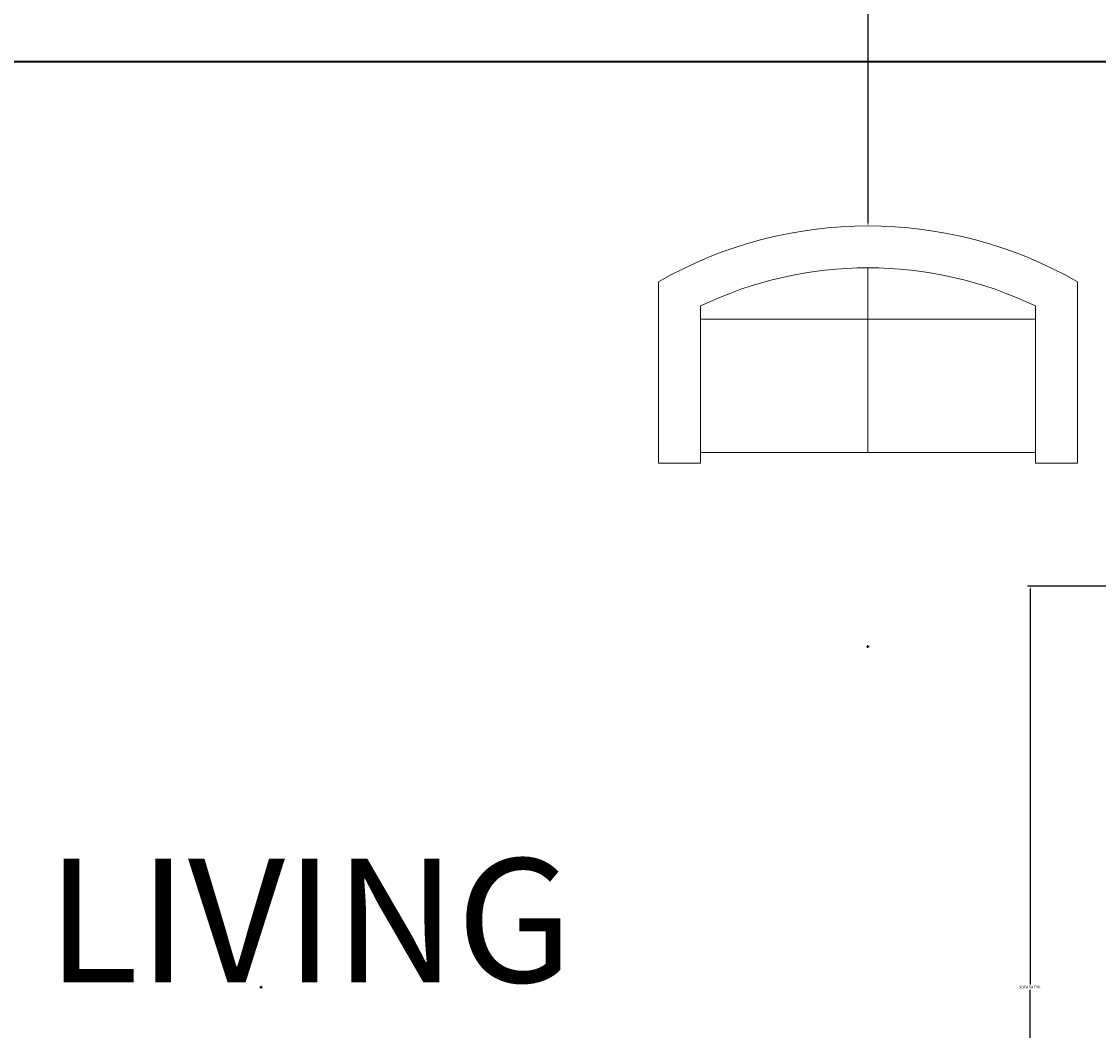
# Model space of a CAD drawing. Units: feet. Extents: x 1654 to 2985, y 1348 to 2230.
# Tile 36 of 53: x 2100 to 2173, y 1821 to 1889. Entities that reach past the tile are written whole.
import ezdxf

# ---------------------------------------------------------------- set-up
doc = ezdxf.new("R2010")
doc.units = ezdxf.units.FT
for name, color, linetype, lineweight in [('A-ANNO-DIMS', 2, 'Continuous', 18), ('A-AREA-IDEN', 7, 'Continuous', 18), ('A-FURN', 8, 'Continuous', 13), ('A-WALL', 7, 'Continuous', 35)]:
    doc.layers.add(name, color=color, linetype=linetype, lineweight=lineweight)
doc.styles.get("Standard").update_dxf_attribs({"font": 'arial.ttf'})
doc.dimstyles.get("Standard").update_dxf_attribs({"dimtxt": 0.18, "dimasz": 0.18, "dimexe": 0.18, "dimexo": 0.0625, "dimgap": 0.09, "dimtad": 0, "dimtih": 1, "dimtoh": 1, "dimdec": 4, "dimzin": 0, "dimdsep": 46, "dimtxsty": 'Standard', "dimcen": 0.09, "dimadec": 0, "dimazin": 0, "dimtfac": 1, "dimtdec": 4, "dimtofl": 0, "dimtmove": 0, "dimatfit": 3, "dimfxl": 1, "dimtolj": 1, "dimtzin": 0, "dimarcsym": 0})

# ---------------------------------------------------------------- blocks, each defined once
blk = doc.blocks.new('Sofa - Roundback Loveseat 5 ft.')
for p, q in [((0, -32.44198), (0, -5.99998)), ((-24, -33.99998), (-24, -11.46958)), ((24.00004, -33.99998), (24.00004, -11.46958)), ((-23.9998, -13.38178), (23.99986, -13.38178)), ((-24, -32.44198), (24.00004, -32.44198))]:
    blk.add_line(p, q)
for points in [[(-24, -33.99998), (-30, -33.99998), (-30, -7.99998)], [(30.00004, -7.99998), (30.00004, -33.99998), (24.00004, -33.99998)]]:
    blk.add_lwpolyline(points)
for centre, radius, start, end in [((0, -60.24998), 60.24998, 60.13715, 119.8628), ((0, -61.38438), 55.38444, 64.32083, 115.6792)]:
    blk.add_arc(centre, radius, start, end)
blk = doc.blocks.new('*D38')
at = {"layer": 'A-ANNO-DIMS', "color": 0, "lineweight": -2, "transparency": 16777216}
for p, q in [((2176.839, 1850.733), (2168.575, 1850.733)), ((2168.755, 1850.553), (2168.755, 1823.764)), ((2168.755, 1796.609), (2168.755, 1823.398)), ((2176.839, 1796.429), (2168.575, 1796.429))]:
    blk.add_line(p, q, dxfattribs=at)
at = {"layer": 'A-ANNO-DIMS', "color": 0, "transparency": 16777216}
for points in [[(2168.725, 1850.553), (2168.785, 1850.553), (2168.755, 1850.733)], [(2168.725, 1796.609), (2168.785, 1796.609), (2168.755, 1796.429)]]:
    blk.add_solid(points, dxfattribs=at)
at = {"layer": 'Defpoints', "color": 0, "transparency": 16777216}
for p in [(2176.901, 1850.733), (2168.755, 1796.429), (2176.901, 1796.429)]:
    blk.add_point(p, dxfattribs=at)
at = {"layer": 'A-ANNO-DIMS', "color": 0, "transparency": 16777216, "insert": (2168.755, 1823.581), "char_height": 0.18, "attachment_point": 5}
blk.add_mtext('\\A1;SOFA 54 TYP.', dxfattribs=at)
blk = doc.blocks.new('*D80')
at = {"layer": 'A-ANNO-DIMS', "color": 0, "lineweight": -2, "transparency": 16777216}
for p, q in [((2070.092, 2039.192), (2070.092, 1534.075)), ((2202.092, 2039.192), (2202.092, 1534.075)), ((2070.272, 1534.255), (2135.813, 1534.255)), ((2201.912, 1534.255), (2136.372, 1534.255))]:
    blk.add_line(p, q, dxfattribs=at)
at = {"layer": 'A-ANNO-DIMS', "color": 0, "transparency": 16777216}
for points in [[(2070.272, 1534.285), (2070.272, 1534.225), (2070.092, 1534.255)], [(2201.912, 1534.285), (2201.912, 1534.225), (2202.092, 1534.255)]]:
    blk.add_solid(points, dxfattribs=at)
at = {"layer": 'Defpoints', "color": 0, "transparency": 16777216}
for p in [(2070.092, 2039.255), (2202.092, 2039.255), (2202.092, 1534.255)]:
    blk.add_point(p, dxfattribs=at)
at = {"layer": 'A-ANNO-DIMS', "color": 0, "transparency": 16777216, "insert": (2136.092, 1534.255), "char_height": 0.18, "attachment_point": 5}
blk.add_mtext('\\A1;132', dxfattribs=at)
blk = doc.blocks.new('*D108')
at = {"layer": 'A-ANNO-DIMS', "color": 0, "lineweight": -2, "transparency": 16777216}
for p, q in [((2116.561, 1823.581), (2116.741, 1823.581)), ((2116.651, 1823.491), (2116.651, 1823.671)), ((2242.014, 1823.581), (2195.183, 1823.581))]:
    blk.add_line(p, q, dxfattribs=at)
at = {"layer": 'A-ANNO-DIMS', "color": 0, "transparency": 16777216}
blk.add_solid([(2195.183, 1823.611), (2195.183, 1823.551), (2195.003, 1823.581)], dxfattribs=at)
at = {"layer": 'Defpoints', "color": 0, "transparency": 16777216}
for p in [(2116.651, 1823.581), (2195.003, 1823.581)]:
    blk.add_point(p, dxfattribs=at)
at = {"layer": 'A-ANNO-DIMS', "color": 0, "transparency": 16777216, "insert": (2242.689, 1823.581), "char_height": 0.18, "attachment_point": 5}
blk.add_mtext('\\A1;2X R78.35', dxfattribs=at)
blk = doc.blocks.new('*D110')
at = {"layer": 'A-ANNO-DIMS', "color": 0, "lineweight": -2, "transparency": 16777216}
for p, q in [((2157.583, 1892.245), (2157.763, 1892.245)), ((2157.763, 1892.245), (2157.763, 1875.33)), ((2157.763, 1846.568), (2157.763, 1846.748)), ((2157.673, 1846.658), (2157.853, 1846.658))]:
    blk.add_line(p, q, dxfattribs=at)
at = {"layer": 'A-ANNO-DIMS', "color": 0, "transparency": 16777216}
blk.add_solid([(2157.793, 1875.33), (2157.733, 1875.33), (2157.763, 1875.15)], dxfattribs=at)
at = {"layer": 'Defpoints', "color": 0, "transparency": 16777216}
for p in [(2157.763, 1875.15), (2157.763, 1846.658)]:
    blk.add_point(p, dxfattribs=at)
at = {"layer": 'A-ANNO-DIMS', "color": 0, "transparency": 16777216, "insert": (2156.908, 1892.245), "char_height": 0.18, "attachment_point": 5}
blk.add_mtext('\\A1;2X R28.49', dxfattribs=at)

msp = doc.modelspace()

# ---------------------------------------------------------------- linework, layer by layer
at = {"layer": 'A-WALL'}
msp.add_line((2202.0924, 1886.2549), (2070.0924, 1886.2549), dxfattribs=at)

# ---------------------------------------------------------------- block references
at = {"layer": 'A-FURN', "xscale": 0.4728872769476647, "yscale": 0.4728872769476647, "zscale": 0.4728872769476647}
msp.add_blockref('Sofa - Roundback Loveseat 5 ft.', (2157.7631, 1875.1496), dxfattribs=at)

# ---------------------------------------------------------------- texts
at = {"layer": 'A-AREA-IDEN'}
msp.add_text('LIVING', height=8.38114, dxfattribs=at).set_placement((2102.1259, 1823.9066))

# ---------------------------------------------------------------- dimensions: what is measured, and where the dimension line sits
at = {"layer": 'A-ANNO-DIMS'}
dim = msp.add_linear_dim(base=(2202.0924, 1534.2549), p1=(2070.0924, 2039.2549), p2=(2202.0924, 2039.2549), dimstyle='Standard', override={"dimdec": 0, "dimlfac": 1, "dimrnd": 0, "dimzin": 0, "dimdsep": 46, "dimlunit": 2}, dxfattribs=at)
dim.commit()
dim.dimension.update_dxf_attribs({"geometry": '*D80', "text_midpoint": (2136.0924, 1534.2549)})
for center, mpoint, picture, middle in [((2157.7631, 1846.6582), (2157.763, 1875.1496), '*D110', (2156.908, 1892.2445)), ((2116.6507, 1823.581), (2195.0027, 1823.581), '*D108', (2242.0138, 1823.581))]:
    dim = msp.add_radius_dim(center=center, mpoint=mpoint, text='2X <>', dimstyle='Standard', override={"dimdec": 2, "dimlfac": 1, "dimrnd": 0, "dimzin": 0, "dimdsep": 46, "dimlunit": 2}, dxfattribs=at)
    dim.commit()
    dim.dimension.update_dxf_attribs({"geometry": picture, "text_midpoint": middle, "dimtype": 164})
dim = msp.add_linear_dim(base=(2168.7554, 1796.4287), p1=(2176.9011, 1850.7334), p2=(2176.9011, 1796.4287), angle=270, text='SOFA <> TYP.', dimstyle='Standard', override={"dimdec": 0, "dimlfac": 1, "dimrnd": 0, "dimzin": 0, "dimdsep": 46, "dimlunit": 2}, dxfattribs=at)
dim.commit()
dim.dimension.update_dxf_attribs({"geometry": '*D38', "text_midpoint": (2168.7554, 1823.5811)})

doc.saveas('drawing.dxf')
